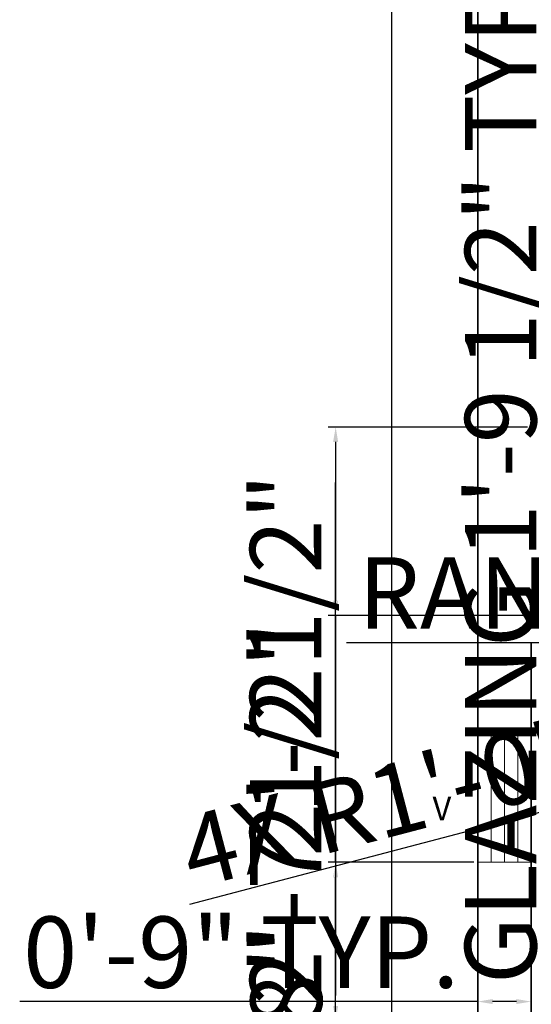
# Model space of a CAD drawing. Units: inches. Extents: x 2691 to 3133, y 1294 to 1993.
# Tile 3 of 7: x 2691 to 2777, y 1696 to 1862. Entities that reach past the tile are written whole.
import ezdxf

# ---------------------------------------------------------------- set-up
doc = ezdxf.new("R2010")
doc.units = ezdxf.units.IN
for name, color, linetype, lineweight in [('A-ANNO-DIMS', 2, 'Continuous', 18), ('A-ANNO-TEXT', 7, 'Continuous', 18), ('A-GLAZ', 4, 'Continuous', 18), ('A-WALL', 7, 'Continuous', 35)]:
    doc.layers.add(name, color=color, linetype=linetype, lineweight=lineweight)
doc.styles.get("Standard").update_dxf_attribs({"font": 'arial.ttf'})
doc.dimstyles.new('ISO-25', dxfattribs={"dimtxt": 12, "dimasz": 2.5, "dimexe": 1.25, "dimexo": 0.625, "dimtad": 1, "dimdec": 1, "dimlunit": 3, "dimtxsty": 'Standard', "dimcen": 2.5, "dimadec": 0, "dimazin": 0, "dimtfac": 1, "dimtdec": 1, "dimtmove": 0, "dimatfit": 3, "dimfxl": 1, "dimarcsym": 0})

# ---------------------------------------------------------------- blocks, each defined once
blk = doc.blocks.new('Window - Wood Frame 36 in. Wide plan')
for p, q in [((0, 6), (0, 0)), ((36, 6), (36, 0)), ((0, 4.5), (36, 4.5)), ((0, 3), (36, 3)), ((0, 1.5), (36, 1.5))]:
    blk.add_line(p, q)
blk = doc.blocks.new('*D11')
at = {"layer": 'A-ANNO-DIMS', "color": 0, "lineweight": -2, "transparency": 16777216}
for p, q in [((2767.62, 1880.05), (2752.52, 1880.05)), ((2753.77, 1877.55), (2753.77, 1426.55)), ((2767.62, 1424.05), (2752.52, 1424.05))]:
    blk.add_line(p, q, dxfattribs=at)
at = {"layer": 'A-ANNO-DIMS', "color": 0, "transparency": 16777216}
for points in [[(2753.35, 1877.55), (2754.18, 1877.55), (2753.77, 1880.05)], [(2753.35, 1426.55), (2754.18, 1426.55), (2753.77, 1424.05)]]:
    blk.add_solid(points, dxfattribs=at)
at = {"layer": 'Defpoints', "color": 0, "transparency": 16777216}
for p in [(2768.25, 1880.05), (2753.77, 1424.05), (2768.25, 1424.05)]:
    blk.add_point(p, dxfattribs=at)
at = {"layer": 'A-ANNO-DIMS', "color": 0, "transparency": 16777216, "insert": (2747.01, 1652.05), "char_height": 12, "attachment_point": 5, "rotation": 90}
blk.add_mtext("38'", dxfattribs=at)
blk = doc.blocks.new('*D18')
at = {"layer": 'A-ANNO-DIMS', "color": 0, "lineweight": -2, "transparency": 16777216}
for p, q in [((2780.49, 1693.45), (2780.49, 1876.36)), ((2777.87, 1693.45), (2781.74, 1693.45)), ((2780.49, 1674.35), (2780.49, 1690.95)), ((2777.87, 1671.85), (2781.74, 1671.85))]:
    blk.add_line(p, q, dxfattribs=at)
at = {"layer": 'A-ANNO-DIMS', "color": 0, "transparency": 16777216}
for points in [[(2780.07, 1690.95), (2780.91, 1690.95), (2780.49, 1693.45)], [(2780.07, 1674.35), (2780.91, 1674.35), (2780.49, 1671.85)]]:
    blk.add_solid(points, dxfattribs=at)
at = {"layer": 'Defpoints', "color": 0, "transparency": 16777216}
for p in [(2777.25, 1693.45), (2780.49, 1693.45), (2777.25, 1671.85)]:
    blk.add_point(p, dxfattribs=at)
at = {"layer": 'A-ANNO-DIMS', "color": 0, "transparency": 16777216, "insert": (2773.66, 1786.16), "char_height": 12, "attachment_point": 5, "rotation": 90}
blk.add_mtext('GLAZING 1\'-9 1/2" TYP.', dxfattribs=at)
blk = doc.blocks.new('*D19')
at = {"layer": 'A-ANNO-DIMS', "color": 0, "lineweight": -2, "transparency": 16777216}
for p, q in [((2768.25, 1694.08), (2768.25, 1697.94)), ((2777.25, 1694.08), (2777.25, 1697.94)), ((2768.25, 1696.69), (2691.35, 1696.69)), ((2774.75, 1696.69), (2770.75, 1696.69))]:
    blk.add_line(p, q, dxfattribs=at)
at = {"layer": 'A-ANNO-DIMS', "color": 0, "transparency": 16777216}
for points in [[(2770.75, 1697.11), (2770.75, 1696.28), (2768.25, 1696.69)], [(2774.75, 1697.11), (2774.75, 1696.28), (2777.25, 1696.69)]]:
    blk.add_solid(points, dxfattribs=at)
at = {"layer": 'Defpoints', "color": 0, "transparency": 16777216}
for p in [(2768.25, 1696.69), (2768.25, 1693.45), (2777.25, 1693.45)]:
    blk.add_point(p, dxfattribs=at)
at = {"layer": 'A-ANNO-DIMS', "color": 0, "transparency": 16777216, "insert": (2728.55, 1703.44), "char_height": 12, "attachment_point": 5}
blk.add_mtext('0\'-9" TYP.', dxfattribs=at)
blk = doc.blocks.new('*D34')
at = {"layer": 'A-ANNO-DIMS', "color": 0, "lineweight": -2, "transparency": 16777216}
for p, q in [((2845.53, 1760.85), (2845.53, 1755.73)), ((2875.53, 1760.85), (2875.53, 1755.73)), ((2845.53, 1756.98), (2746.23, 1756.98)), ((2873.03, 1756.98), (2848.03, 1756.98))]:
    blk.add_line(p, q, dxfattribs=at)
at = {"layer": 'A-ANNO-DIMS', "color": 0, "transparency": 16777216}
for points in [[(2848.03, 1757.39), (2848.03, 1756.56), (2845.53, 1756.98)], [(2873.03, 1757.39), (2873.03, 1756.56), (2875.53, 1756.98)]]:
    blk.add_solid(points, dxfattribs=at)
at = {"layer": 'Defpoints', "color": 0, "transparency": 16777216}
for p in [(2845.53, 1761.48), (2875.53, 1761.48), (2845.53, 1756.98)]:
    blk.add_point(p, dxfattribs=at)
at = {"layer": 'A-ANNO-DIMS', "color": 0, "transparency": 16777216, "insert": (2794.63, 1763.81), "char_height": 12, "attachment_point": 5}
blk.add_mtext('RANGE 2\'-6"', dxfattribs=at)
blk = doc.blocks.new('*D45')
at = {"layer": 'A-ANNO-DIMS', "color": 0, "lineweight": -2, "transparency": 16777216}
for p, q in [((2744.4, 1671.85), (2744.4, 1707.71)), ((2767.62, 1671.85), (2743.15, 1671.85)), ((2744.4, 1642.55), (2744.4, 1669.35)), ((2776.62, 1640.05), (2743.15, 1640.05))]:
    blk.add_line(p, q, dxfattribs=at)
at = {"layer": 'A-ANNO-DIMS', "color": 0, "transparency": 16777216}
for points in [[(2743.98, 1669.35), (2744.82, 1669.35), (2744.4, 1671.85)], [(2743.98, 1642.55), (2744.82, 1642.55), (2744.4, 1640.05)]]:
    blk.add_solid(points, dxfattribs=at)
at = {"layer": 'Defpoints', "color": 0, "transparency": 16777216}
for p in [(2744.4, 1671.85), (2768.25, 1671.85), (2777.25, 1640.05)]:
    blk.add_point(p, dxfattribs=at)
at = {"layer": 'A-ANNO-DIMS', "color": 0, "transparency": 16777216, "insert": (2737.65, 1691.03), "char_height": 12, "attachment_point": 5, "rotation": 90}
blk.add_mtext('2\'-8"', dxfattribs=at)
blk = doc.blocks.new('*D46')
at = {"layer": 'A-ANNO-DIMS', "color": 0, "lineweight": -2, "transparency": 16777216}
for p, q in [((2744.4, 1720.1), (2744.4, 1783.91)), ((2767.62, 1720.1), (2743.15, 1720.1)), ((2744.4, 1695.95), (2744.4, 1717.6)), ((2767.62, 1693.45), (2743.15, 1693.45))]:
    blk.add_line(p, q, dxfattribs=at)
at = {"layer": 'A-ANNO-DIMS', "color": 0, "transparency": 16777216}
for points in [[(2743.98, 1717.6), (2744.82, 1717.6), (2744.4, 1720.1)], [(2743.98, 1695.95), (2744.82, 1695.95), (2744.4, 1693.45)]]:
    blk.add_solid(points, dxfattribs=at)
at = {"layer": 'Defpoints', "color": 0, "transparency": 16777216}
for p in [(2744.4, 1720.1), (2768.25, 1720.1), (2768.25, 1693.45)]:
    blk.add_point(p, dxfattribs=at)
at = {"layer": 'A-ANNO-DIMS', "color": 0, "transparency": 16777216, "insert": (2737.57, 1753.25), "char_height": 12, "attachment_point": 5, "rotation": 90}
blk.add_mtext('2\'-2 1/2"', dxfattribs=at)
blk = doc.blocks.new('*D59')
at = {"layer": 'A-ANNO-DIMS', "color": 0, "lineweight": -2, "transparency": 16777216}
for p, q in [((2776.62, 1793.25), (2743.15, 1793.25)), ((2744.4, 1790.75), (2744.4, 1764.05)), ((2776.62, 1761.55), (2743.15, 1761.55)), ((2744.4, 1761.55), (2744.4, 1697.74))]:
    blk.add_line(p, q, dxfattribs=at)
at = {"layer": 'A-ANNO-DIMS', "color": 0, "transparency": 16777216}
for points in [[(2743.98, 1790.75), (2744.82, 1790.75), (2744.4, 1793.25)], [(2743.98, 1764.05), (2744.82, 1764.05), (2744.4, 1761.55)]]:
    blk.add_solid(points, dxfattribs=at)
at = {"layer": 'Defpoints', "color": 0, "transparency": 16777216}
for p in [(2777.25, 1793.25), (2744.4, 1761.55), (2777.25, 1761.55)]:
    blk.add_point(p, dxfattribs=at)
at = {"layer": 'A-ANNO-DIMS', "color": 0, "transparency": 16777216, "insert": (2737.57, 1728.4), "char_height": 12, "attachment_point": 5, "rotation": 90}
blk.add_mtext('2\'-7 1/2"', dxfattribs=at)
blk = doc.blocks.new('*D68')
at = {"layer": 'A-ANNO-DIMS', "color": 0, "lineweight": -2, "transparency": 16777216}
for p, q in [((2805.12, 1735.47), (2793.35, 1732.38)), ((2719.94, 1713.09), (2790.93, 1731.75))]:
    blk.add_line(p, q, dxfattribs=at)
at = {"layer": 'A-ANNO-DIMS', "color": 0, "transparency": 16777216}
blk.add_solid([(2790.82, 1732.15), (2791.03, 1731.34), (2793.35, 1732.38)], dxfattribs=at)
at = {"layer": 'Defpoints', "color": 0, "transparency": 16777216}
for p in [(2805.12, 1735.47), (2793.35, 1732.38)]:
    blk.add_point(p, dxfattribs=at)
at = {"layer": 'A-ANNO-DIMS', "color": 0, "transparency": 16777216, "insert": (2752.51, 1728.63), "char_height": 12, "attachment_point": 5, "rotation": 14.721}
blk.add_mtext('4X R1\'-0"', dxfattribs=at)

msp = doc.modelspace()

# ---------------------------------------------------------------- linework, layer by layer
at = {"layer": 'A-WALL'}
for p, q in [((2768.25, 1880.05), (2768.25, 1424.05)), ((2777.25, 1757.05), (2777.25, 1644.55))]:
    msp.add_line(p, q, dxfattribs=at)

# ---------------------------------------------------------------- block references
at = {"layer": 'A-GLAZ', "xscale": 0.6, "yscale": 1.5, "rotation": 90}
msp.add_blockref('Window - Wood Frame 36 in. Wide plan', (2777.25, 1720.1), dxfattribs=at)

# ---------------------------------------------------------------- texts
at = {"layer": 'A-ANNO-TEXT', "insert": (2760.67, 1731.13), "char_height": 4, "attachment_point": 1}
msp.add_mtext_dynamic_manual_height_columns('V', width=0.1038, gutter_width=12.5, heights=[0], dxfattribs=at)

# ---------------------------------------------------------------- dimensions: what is measured, and where the dimension line sits
at = {"layer": 'A-ANNO-DIMS'}
for base, p1, p2, override, picture, middle in [((2753.77, 1424.05), (2768.25, 1880.05), (2768.25, 1424.05), {"dimclrd": 0, "dimclre": 0, "dimclrt": 0}, '*D11', (2747.01, 1652.05)), ((2744.4, 1761.55), (2777.25, 1793.25), (2777.25, 1761.55), {"dimdec": 1, "dimlfac": 1, "dimrnd": 0, "dimzin": 1, "dimdsep": 46, "dimlunit": 4, "dimfrac": 2}, '*D59', (2737.57, 1728.4)), ((2744.3996, 1720.0971), (2768.2496, 1693.4519), (2768.2496, 1720.0971), {"dimdec": 1, "dimlfac": 1, "dimrnd": 0, "dimzin": 1, "dimdsep": 46, "dimlunit": 4, "dimfrac": 2}, '*D46', (2737.5699, 1753.2548)), ((2744.4, 1671.85), (2777.25, 1640.05), (2768.25, 1671.85), {"dimdec": 1, "dimlfac": 1, "dimrnd": 0, "dimzin": 1, "dimdsep": 46, "dimlunit": 4, "dimfrac": 2}, '*D45', (2737.65, 1691.03))]:
    dim = msp.add_linear_dim(base=base, p1=p1, p2=p2, angle=90, dimstyle='ISO-25', override=override, dxfattribs=at)
    dim.commit()
    dim.dimension.update_dxf_attribs({"geometry": picture, "text_midpoint": middle})
for base, p1, p2, angle, text, picture, middle in [((2780.49, 1693.45), (2777.25, 1671.85), (2777.25, 1693.45), 90, 'GLAZING <> TYP.', '*D18', (2773.66, 1786.16)), ((2845.53, 1756.98), (2875.53, 1761.48), (2845.53, 1761.48), 180, 'RANGE <>', '*D34', (2794.63, 1763.81)), ((2768.25, 1696.69), (2777.25, 1693.45), (2768.25, 1693.45), 180, '<> TYP.', '*D19', (2728.55, 1703.44))]:
    dim = msp.add_linear_dim(base=base, p1=p1, p2=p2, angle=angle, text=text, dimstyle='ISO-25', override={"dimdec": 1, "dimlfac": 1, "dimrnd": 0, "dimzin": 1, "dimdsep": 46, "dimlunit": 4, "dimfrac": 2}, dxfattribs=at)
    dim.commit()
    dim.dimension.update_dxf_attribs({"geometry": picture, "text_midpoint": middle})
dim = msp.add_radius_dim(center=(2805.12, 1735.47), mpoint=(2793.35, 1732.38), text='4X <>', dimstyle='ISO-25', override={"dimdec": 1, "dimlfac": 1, "dimrnd": 0, "dimzin": 1, "dimdsep": 46, "dimlunit": 4, "dimfrac": 2}, dxfattribs=at)
dim.commit()
dim.dimension.update_dxf_attribs({"geometry": '*D68', "text_midpoint": (2752.51, 1728.63)})

doc.saveas('drawing.dxf')
